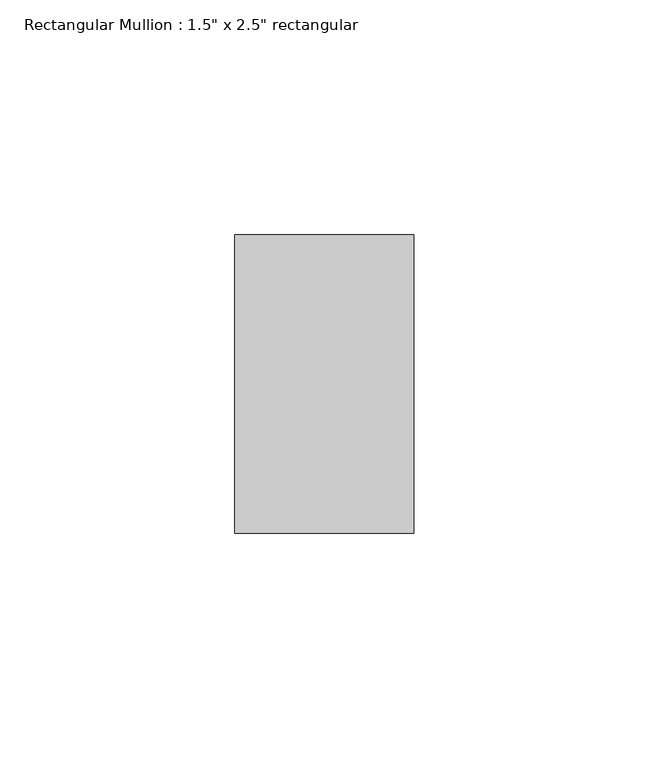
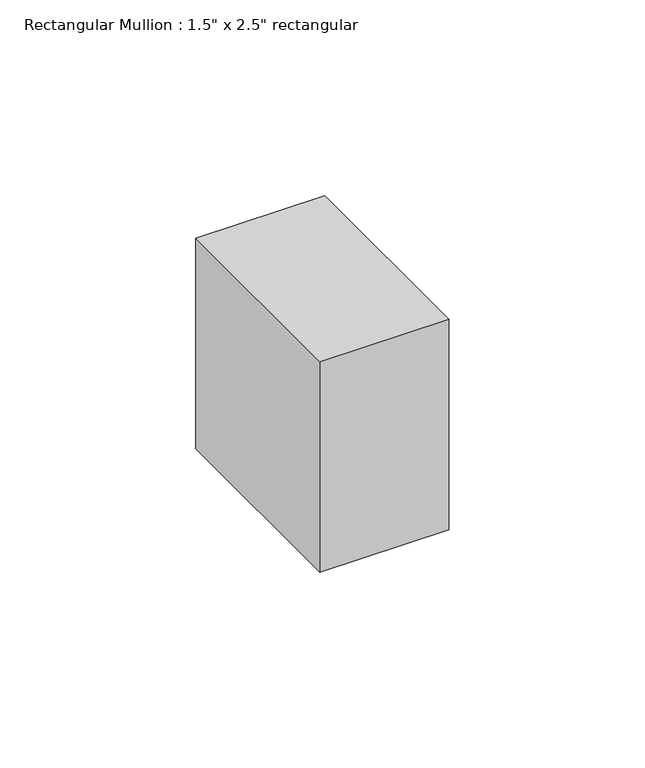
"""IFC4 building model written with IfcOpenShell, lengths in millimetres: member geometry."""

from ifc_helpers import new_model, si_unit, frame, origin, place, context, project, spatial, polyline, outline, extrude, source, transform, mapped, element, save


def member_1ff0c156(model_context):
    return source(origin(), model_context, "Body", "SweptSolid", [
        extrude(outline(polyline([(19.05, 31.75), (19.05, -31.75), (-19.05, -31.75), (-19.05, 31.75), (19.05, 31.75)])), frame((0.0, 0.0, -65.7159256), z_axis=(0.0, 0.0, 1.0), x_axis=(1.0, 0.0, 0.0)), (0.0, 0.0, 1.0), 65.7159256),
    ])


if __name__ == "__main__":
    model = new_model("IFC4")
    model_context = context("Model", 3, world=origin())
    ifc_project = project(units=[si_unit("LENGTHUNIT", "METRE", prefix="MILLI")], contexts=[model_context])
    site = spatial("IfcSite", under=ifc_project)
    building = spatial("IfcBuilding", under=site)
    placement = place(None, origin())
    member_shape = member_1ff0c156(model_context)
    element("IfcMember", 1, ObjectType="Rectangular Mullion : 1.5\" x 2.5\" rectangular", at=placement, inside=building, context=model_context, shape_type="MappedRepresentation", body=[
        mapped(member_shape, transform((0.0, 0.0, 0.0), x_axis=(1.0, 0.0, 0.0), y_axis=(0.0, 1.0, 0.0), z_axis=(0.0, 0.0, 1.0))),
    ])
    save(model, "model.ifc")

# Revit data of these elements
# Type "Rectangular Mullion : 1.5\" x 2.5\" rectangular"
#   built-in parameter 1007304 = 0.208333 (stored number, unit not read)
#   built-in parameter 1007301 = 0.0625 (stored number, unit not read)
#   built-in parameter 1007300 = 0.0625 (stored number, unit not read)
